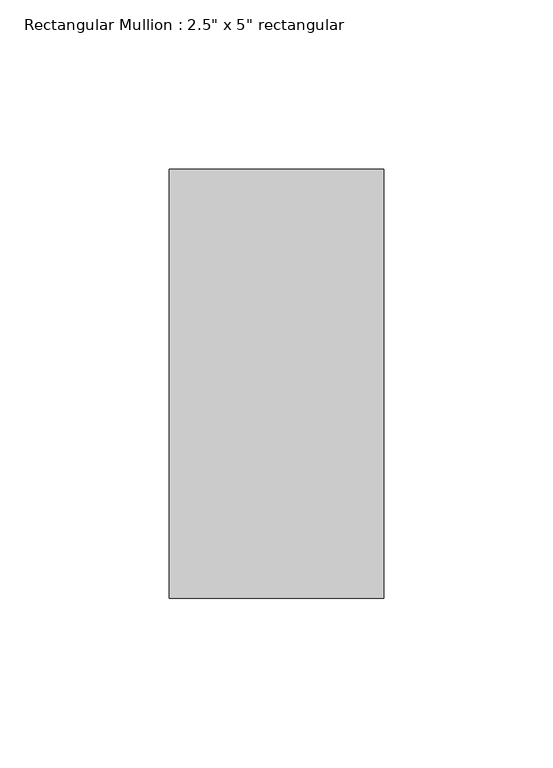
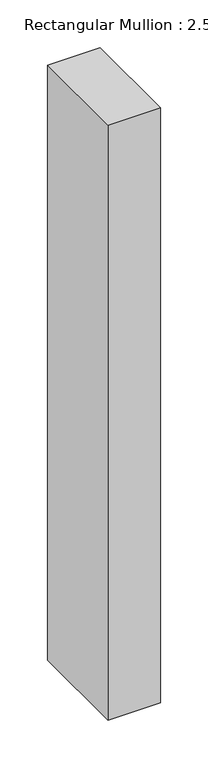
"""IFC4 building model written with IfcOpenShell, lengths in millimetres: member geometry."""

from ifc_helpers import new_model, si_unit, frame, origin, place, context, project, spatial, polyline, outline, extrude, source, transform, mapped, element, save


def member_61742b2b(model_context):
    return source(origin(), model_context, "Body", "SweptSolid", [
        extrude(outline(polyline([(31.75, 63.5), (31.75, -63.5), (-31.75, -63.5), (-31.75, 63.5), (31.75, 63.5)])), frame((0.0, 0.0, -762.0), z_axis=(0.0, 0.0, 1.0), x_axis=(1.0, 0.0, 0.0)), (0.0, 0.0, 1.0), 762.0),
    ])


if __name__ == "__main__":
    model = new_model("IFC4")
    model_context = context("Model", 3, world=origin())
    ifc_project = project(units=[si_unit("LENGTHUNIT", "METRE", prefix="MILLI")], contexts=[model_context])
    site = spatial("IfcSite", under=ifc_project)
    building = spatial("IfcBuilding", under=site)
    placement = place(None, origin())
    member_shape = member_61742b2b(model_context)
    element("IfcMember", 1, ObjectType="Rectangular Mullion : 2.5\" x 5\" rectangular", at=placement, inside=building, context=model_context, shape_type="MappedRepresentation", body=[
        mapped(member_shape, transform((0.0, 0.0, 0.0), x_axis=(1.0, 0.0, 0.0), y_axis=(0.0, 1.0, 0.0), z_axis=(0.0, 0.0, 1.0))),
    ])
    save(model, "model.ifc")

# Revit data of these elements
# Type "Rectangular Mullion : 2.5\" x 5\" rectangular"
#   built-in parameter 1007304 = 0.416667 (stored number, unit not read)
#   built-in parameter 1007301 = 0.104167 (stored number, unit not read)
#   built-in parameter 1007300 = 0.104167 (stored number, unit not read)
# Element 1 (IfcMember, "Rectangular Mullion : 2.5\" x 5\" rectangular")
#   Materials on its faces: "Aluminum"
# Materials
#   "Aluminum": class "Metal", colour RGB 247 247 247, transparency 0, Description = "Aluminum 6061", Cost = 0
